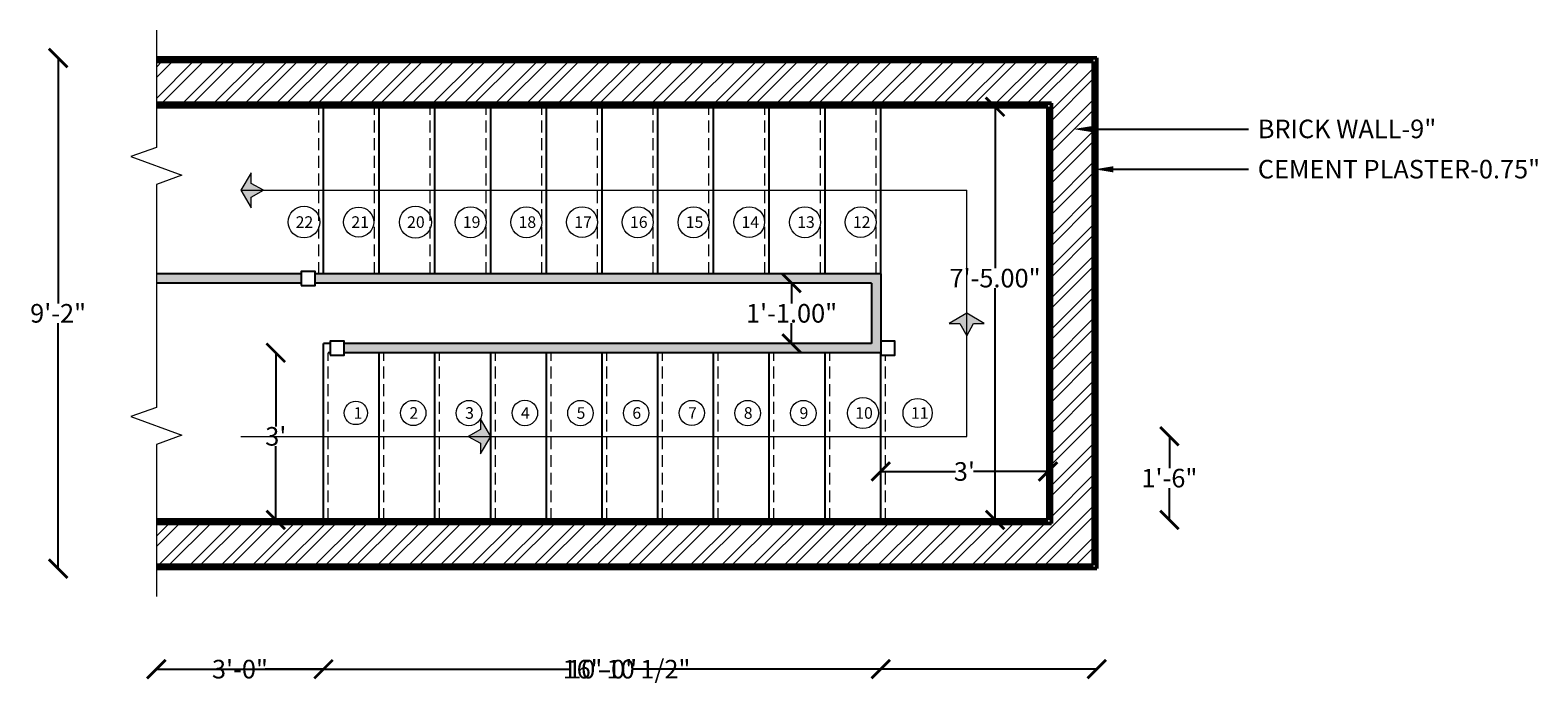
# Model space of a CAD drawing. Units: inches. Extents: x -27 to 693, y -28 to 216.
# Tile 1 of 2: x -27 to 298, y -28 to 116. Entities that reach past the tile are written whole.
import ezdxf
from ezdxf import colors
from ezdxf.entities.mleader import LeaderData, LeaderLine
from ezdxf.math import Vec2, Vec3

# ---------------------------------------------------------------- set-up
doc = ezdxf.new("R2010")
doc.units = ezdxf.units.IN
doc.linetypes.add('DASHED', pattern=[19.05, 12.7, -6.35])
for name, color, linetype, lineweight in [('A-ANNO-DIMS', 2, 'Continuous', 18), ('A-ANNO-SYMB', 3, 'Continuous', 18), ('A-ANNO-TEXT', 7, 'Continuous', 18), ('A-FLOR-HRAL', 4, 'Continuous', 25), ('A-FLOR-PATT', 8, 'Continuous', 13), ('A-FLOR-STRS', 1, 'Continuous', 25), ('A-FLOR-STRS-OVHD', 1, 'DASHED', 18), ('A-WALL', 7, 'Continuous', 50), ('A-WALL-PATT', 8, 'Continuous', 18)]:
    doc.layers.add(name, color=color, linetype=linetype, lineweight=lineweight)
doc.styles.get("Standard").update_dxf_attribs({"font": 'arial.ttf'})
doc.dimstyles.get("Standard").update_dxf_attribs({"dimtxt": 4, "dimasz": 4, "dimexe": 0.18, "dimexo": 0.0625, "dimgap": 0.09, "dimtad": 0, "dimtih": 1, "dimtoh": 1, "dimzin": 0, "dimdsep": 46, "dimlunit": 3, "dimtxsty": 'Standard', "dimblk": 'ARCHTICK', "dimcen": 0.09, "dimse1": 1, "dimse2": 1, "dimclrd": 4, "dimclrt": 2, "dimadec": 0, "dimazin": 0, "dimtfac": 1, "dimtofl": 0, "dimtmove": 0, "dimatfit": 3, "dimfxl": 1, "dimtolj": 1, "dimtzin": 0, "dimarcsym": 0})

# ---------------------------------------------------------------- blocks, each defined once
blk = doc.blocks.new('_ArchTick')
at = {"color": 0, "linetype": 'ByBlock', "const_width": 0.15}
blk.add_lwpolyline([(-0.5, -0.5), (0.5, 0.5)], dxfattribs=at)
blk = doc.blocks.new('*D3')
at = {"layer": 'A-ANNO-DIMS', "color": 0, "lineweight": -2, "transparency": 16777216}
for p, q in [((25.74, 46.24), (25.74, 30.37)), ((25.74, 10.24), (25.74, 26.1))]:
    blk.add_line(p, q, dxfattribs=at)
at = {"layer": 'DEFPOINTS', "color": 0, "transparency": 16777216}
for p in [(25.74, 46.24), (48.02, 46.24), (48.02, 10.24)]:
    blk.add_point(p, dxfattribs=at)
at = {"layer": 'A-ANNO-DIMS', "color": 0, "lineweight": -2, "transparency": 16777216, "xscale": 4, "yscale": 4, "zscale": 4}
for p, rotation in [((25.74, 46.24), 90), ((25.74, 10.24), 270)]:
    blk.add_blockref('_ArchTick', p, dxfattribs=dict(at, rotation=rotation))
at = {"layer": 'A-ANNO-DIMS', "color": 0, "transparency": 16777216, "insert": (25.74, 28.24), "char_height": 4, "attachment_point": 5}
blk.add_mtext("\\A1;3'", dxfattribs=at)
blk = doc.blocks.new('*D4')
at = {"layer": 'A-ANNO-DIMS', "color": 0, "lineweight": -2, "transparency": 16777216}
for p, q in [((136.81, 61.24), (136.81, 56.87)), ((136.81, 48.24), (136.81, 52.6))]:
    blk.add_line(p, q, dxfattribs=at)
at = {"layer": 'DEFPOINTS', "color": 0, "transparency": 16777216}
for p in [(154.02, 61.24), (136.81, 48.24), (154.02, 48.24)]:
    blk.add_point(p, dxfattribs=at)
at = {"layer": 'A-ANNO-DIMS', "color": 0, "lineweight": -2, "transparency": 16777216, "xscale": 4, "yscale": 4, "zscale": 4}
for p, rotation in [((136.81, 61.24), 90), ((136.81, 48.24), 270)]:
    blk.add_blockref('_ArchTick', p, dxfattribs=dict(at, rotation=rotation))
at = {"layer": 'A-ANNO-DIMS', "color": 0, "transparency": 16777216, "insert": (136.81, 54.74), "char_height": 4, "attachment_point": 5}
blk.add_mtext('\\A1;1\'-1.00"', dxfattribs=at)
blk = doc.blocks.new('*D5')
at = {"layer": 'A-ANNO-DIMS', "color": 0, "lineweight": -2, "transparency": 16777216}
for p, q in [((180.62, 99.24), (180.62, 64.45)), ((180.62, 10.24), (180.62, 60.18))]:
    blk.add_line(p, q, dxfattribs=at)
at = {"layer": 'DEFPOINTS', "color": 0, "transparency": 16777216}
for p in [(180.62, 99.24), (192.02, 99.24), (192.02, 10.24)]:
    blk.add_point(p, dxfattribs=at)
at = {"layer": 'A-ANNO-DIMS', "color": 0, "lineweight": -2, "transparency": 16777216, "xscale": 4, "yscale": 4, "zscale": 4}
for p, rotation in [((180.62, 99.24), 90), ((180.62, 10.24), 270)]:
    blk.add_blockref('_ArchTick', p, dxfattribs=dict(at, rotation=rotation))
at = {"layer": 'A-ANNO-DIMS', "color": 0, "transparency": 16777216, "insert": (180.62, 62.32), "char_height": 4, "attachment_point": 5}
blk.add_mtext('\\A1;7\'-5.00"', dxfattribs=at)
blk = doc.blocks.new('*D6')
at = {"layer": 'A-ANNO-DIMS', "color": 0, "lineweight": -2, "transparency": 16777216}
for p, q in [((156.02, 20.67), (172.09, 20.67)), ((192.02, 20.67), (175.95, 20.67))]:
    blk.add_line(p, q, dxfattribs=at)
at = {"layer": 'DEFPOINTS', "color": 0, "transparency": 16777216}
for p in [(192.02, 20.67), (156.02, 10.24), (192.02, 10.24)]:
    blk.add_point(p, dxfattribs=at)
at = {"layer": 'A-ANNO-DIMS', "color": 0, "lineweight": -2, "transparency": 16777216, "xscale": 4, "yscale": 4, "zscale": 4, "rotation": 180}
blk.add_blockref('_ArchTick', (156.02, 20.67), dxfattribs=at)
at = {"layer": 'A-ANNO-DIMS', "color": 0, "lineweight": -2, "transparency": 16777216, "xscale": 4, "yscale": 4, "zscale": 4}
blk.add_blockref('_ArchTick', (192.02, 20.67), dxfattribs=at)
at = {"layer": 'A-ANNO-DIMS', "color": 0, "transparency": 16777216, "insert": (174.02, 20.67), "char_height": 4, "attachment_point": 5}
blk.add_mtext("\\A1;3'", dxfattribs=at)
blk = doc.blocks.new('*D11')
at = {"layer": 'A-ANNO-DIMS', "color": 4, "lineweight": -2, "transparency": 16777216}
for p, q in [((0.02, -21.91), (88.28, -21.91)), ((202.52, -21.91), (114.25, -21.91))]:
    blk.add_line(p, q, dxfattribs=at)
at = {"layer": 'DEFPOINTS', "color": 0, "transparency": 16777216}
for p in [(0.02, -0.26), (202.52, -0.26), (202.52, -21.91)]:
    blk.add_point(p, dxfattribs=at)
at = {"layer": 'A-ANNO-DIMS', "color": 4, "lineweight": -2, "transparency": 16777216, "xscale": 4, "yscale": 4, "zscale": 4, "rotation": 180}
blk.add_blockref('_ArchTick', (0.02, -21.91), dxfattribs=at)
at = {"layer": 'A-ANNO-DIMS', "color": 4, "lineweight": -2, "transparency": 16777216, "xscale": 4, "yscale": 4, "zscale": 4}
blk.add_blockref('_ArchTick', (202.52, -21.91), dxfattribs=at)
at = {"layer": 'A-ANNO-DIMS', "color": 2, "transparency": 16777216, "insert": (101.27, -21.91), "char_height": 4, "attachment_point": 5}
blk.add_mtext('\\A1;16\'-10 1/2"', dxfattribs=at)
blk = doc.blocks.new('*D12')
at = {"layer": 'A-ANNO-DIMS', "color": 4, "lineweight": -2, "transparency": 16777216}
for p, q in [((0.02, -21.91), (12.61, -21.91)), ((36.02, -21.91), (23.42, -21.91))]:
    blk.add_line(p, q, dxfattribs=at)
at = {"layer": 'DEFPOINTS', "color": 0, "transparency": 16777216}
for p in [(0.02, 10.24), (36.02, 10.24), (36.02, -21.91)]:
    blk.add_point(p, dxfattribs=at)
at = {"layer": 'A-ANNO-DIMS', "color": 4, "lineweight": -2, "transparency": 16777216, "xscale": 4, "yscale": 4, "zscale": 4, "rotation": 180}
blk.add_blockref('_ArchTick', (0.02, -21.91), dxfattribs=at)
at = {"layer": 'A-ANNO-DIMS', "color": 4, "lineweight": -2, "transparency": 16777216, "xscale": 4, "yscale": 4, "zscale": 4}
blk.add_blockref('_ArchTick', (36.02, -21.91), dxfattribs=at)
at = {"layer": 'A-ANNO-DIMS', "color": 2, "transparency": 16777216, "insert": (18.02, -21.91), "char_height": 4, "attachment_point": 5}
blk.add_mtext('\\A1;3\'-0"', dxfattribs=at)
blk = doc.blocks.new('*D13')
at = {"layer": 'A-ANNO-DIMS', "color": 4, "lineweight": -2, "transparency": 16777216}
for p, q in [((36.02, -21.91), (89.24, -21.91)), ((156.02, -21.91), (102.79, -21.91))]:
    blk.add_line(p, q, dxfattribs=at)
at = {"layer": 'DEFPOINTS', "color": 0, "transparency": 16777216}
for p in [(36.02, 10.24), (156.02, 10.24), (156.02, -21.91)]:
    blk.add_point(p, dxfattribs=at)
at = {"layer": 'A-ANNO-DIMS', "color": 4, "lineweight": -2, "transparency": 16777216, "xscale": 4, "yscale": 4, "zscale": 4, "rotation": 180}
blk.add_blockref('_ArchTick', (36.02, -21.91), dxfattribs=at)
at = {"layer": 'A-ANNO-DIMS', "color": 4, "lineweight": -2, "transparency": 16777216, "xscale": 4, "yscale": 4, "zscale": 4}
blk.add_blockref('_ArchTick', (156.02, -21.91), dxfattribs=at)
at = {"layer": 'A-ANNO-DIMS', "color": 2, "transparency": 16777216, "insert": (96.02, -21.91), "char_height": 4, "attachment_point": 5}
blk.add_mtext('\\A1;10\'-0"', dxfattribs=at)
blk = doc.blocks.new('*D14')
at = {"layer": 'A-ANNO-DIMS', "color": 4, "lineweight": -2, "transparency": 16777216}
for p, q in [((-21.13, 109.74), (-21.13, 56.87)), ((-21.13, -0.26), (-21.13, 52.6))]:
    blk.add_line(p, q, dxfattribs=at)
at = {"layer": 'DEFPOINTS', "color": 0, "transparency": 16777216}
for p in [(-21.13, 109.74), (0.02, 109.74), (0.02, -0.26)]:
    blk.add_point(p, dxfattribs=at)
at = {"layer": 'A-ANNO-DIMS', "color": 4, "lineweight": -2, "transparency": 16777216, "xscale": 4, "yscale": 4, "zscale": 4}
for p, rotation in [((-21.13, 109.74), 90), ((-21.13, -0.26), 270)]:
    blk.add_blockref('_ArchTick', p, dxfattribs=dict(at, rotation=rotation))
at = {"layer": 'A-ANNO-DIMS', "color": 2, "transparency": 16777216, "insert": (-21.13, 54.74), "char_height": 4, "attachment_point": 5}
blk.add_mtext('\\A1;9\'-2"', dxfattribs=at)
blk = doc.blocks.new('*D15')
at = {"layer": 'A-ANNO-DIMS', "color": 4, "lineweight": -2, "transparency": 16777216}
for p, q in [((218.17, 28.24), (218.17, 21.37)), ((218.17, 10.24), (218.17, 17.1))]:
    blk.add_line(p, q, dxfattribs=at)
at = {"layer": 'DEFPOINTS', "color": 0, "transparency": 16777216}
for p in [(174.52, 28.24), (192.02, 10.24), (218.17, 10.24)]:
    blk.add_point(p, dxfattribs=at)
at = {"layer": 'A-ANNO-DIMS', "color": 4, "lineweight": -2, "transparency": 16777216, "xscale": 4, "yscale": 4, "zscale": 4}
for p, rotation in [((218.17, 28.24), 90), ((218.17, 10.24), 270)]:
    blk.add_blockref('_ArchTick', p, dxfattribs=dict(at, rotation=rotation))
at = {"layer": 'A-ANNO-DIMS', "color": 2, "transparency": 16777216, "insert": (218.17, 19.24), "char_height": 4, "attachment_point": 5}
blk.add_mtext('\\A1;1\'-6"', dxfattribs=at)

msp = doc.modelspace()

# ---------------------------------------------------------------- hatches: boundary and pattern name
at = {"layer": 'A-ANNO-SYMB'}
h = msp.add_hatch(color=256, dxfattribs=at)
h.dxf.hatch_style = 1
h.paths.add_polyline_path([(20.411, 77.497), (20.411, 79.771), (23.089, 81.237), (18.209, 81.237)])
h.paths.add_polyline_path([(18.209, 81.237), (23.089, 81.237), (20.411, 82.703), (20.411, 84.977)])
h = msp.add_hatch(color=256, dxfattribs=at)
h.dxf.hatch_style = 1
h.paths.add_polyline_path([(170.776, 52.535), (173.051, 52.535), (174.517, 49.857), (174.517, 54.737)])
h.paths.add_polyline_path([(174.517, 54.737), (174.517, 49.857), (175.982, 52.535), (178.257, 52.535)])
h = msp.add_hatch(color=256, dxfattribs=at)
h.dxf.hatch_style = 1
h.paths.add_polyline_path([(69.814, 31.977), (69.814, 29.703), (67.136, 28.237), (72.017, 28.237)])
h.paths.add_polyline_path([(72.017, 28.237), (67.136, 28.237), (69.814, 26.771), (69.814, 24.497)])
at = {"layer": 'A-FLOR-PATT'}
h = msp.add_hatch(dxfattribs=at)
h.set_pattern_fill('GOST_GLASS', color=256, scale=0.2)
h.paths.add_polyline_path([(156.017, 63.237), (34.183, 63.237), (34.183, 61.237), (154.017, 61.237), (154.017, 48.237), (40.433, 48.237), (40.433, 46.237), (156.017, 46.237)])
h.paths.add_polyline_path([(31.183, 63.237), (0.017, 63.237), (0.017, 61.237), (31.183, 61.237)])
at = {"layer": 'A-WALL-PATT'}
h = msp.add_hatch(dxfattribs=at)
h.set_pattern_fill('AR-CONC', color=256, scale=0.01)
h.paths.add_polyline_path([(192.767, 99.987), (0.017, 99.987), (0.017, 99.237), (192.017, 99.237), (192.017, 10.237), (0.017, 10.237), (0.017, 9.487), (192.767, 9.487)], flags=17)
h.paths.add_polyline_path([(202.517, 109.737), (0.017, 109.737), (0.017, 108.987), (201.767, 108.987), (201.767, 0.487), (0.017, 0.487), (0.017, -0.263), (202.517, -0.263)])
h = msp.add_hatch(dxfattribs=at)
h.set_pattern_fill('ANSI32', color=256, scale=0.5)
h.paths.add_polyline_path([(201.767, 108.987), (0.017, 108.987), (0.017, 99.987), (192.767, 99.987), (192.767, 9.487), (0.017, 9.487), (0.017, 0.487), (201.767, 0.487)])

# ---------------------------------------------------------------- linework, layer by layer
at = {"layer": 'A-ANNO-SYMB'}
for p, q in [((18.209, 81.237), (174.517, 81.237)), ((174.517, 28.237), (174.517, 81.237)), ((18.209, 28.237), (174.517, 28.237))]:
    msp.add_line(p, q, dxfattribs=at)
for points in [[(0.017, 115.737), (0.017, 90.487), (-5.478, 88.487), (5.512, 84.487), (0.017, 82.487), (0.017, 57.237)], [(0.017, 67.237), (0.017, 34.487), (-5.478, 32.487), (5.512, 28.487), (0.017, 26.487), (0.017, -6.263)]]:
    msp.add_lwpolyline(points, dxfattribs=at)
for points in [[(23.089, 81.237), (20.411, 82.703), (20.411, 84.977), (18.209, 81.237), (20.411, 77.497), (20.411, 79.771)], [(174.517, 49.857), (175.982, 52.535), (178.257, 52.535), (174.517, 54.737), (170.776, 52.535), (173.051, 52.535)], [(67.136, 28.237), (69.814, 26.771), (69.814, 24.497), (72.017, 28.237), (69.814, 31.977), (69.814, 29.703)]]:
    msp.add_lwpolyline(points, close=True, dxfattribs=at)
for centre, radius in [((31.816, 74.385), 3.419), ((43.587, 74.385), 3.243), ((55.824, 74.364), 3.439), ((67.692, 74.364), 3.337), ((79.692, 74.364), 3.337), ((91.69, 74.385), 3.321), ((103.689, 74.364), 3.334), ((115.699, 74.364), 3.342), ((127.684, 74.385), 3.317), ((139.69, 74.363), 3.335), ((151.677, 74.385), 3.311), ((42.977, 33.268), 2.514), ((55.345, 33.268), 2.727), ((67.335, 33.246), 2.739), ((79.381, 33.273), 2.746), ((91.345, 33.252), 2.74), ((103.342, 33.246), 2.742), ((115.326, 33.273), 2.711), ((127.34, 33.246), 2.741), ((139.339, 33.246), 2.74), ((152.185, 33.246), 3.331), ((163.948, 33.268), 3.14)]:
    msp.add_circle(centre, radius, dxfattribs=at)
at = {"layer": 'A-FLOR-HRAL'}
for p, q in [((31.183, 63.237), (0.017, 63.237)), ((156.017, 63.237), (34.183, 63.237)), ((156.017, 63.237), (156.017, 46.237)), ((31.183, 61.237), (0.017, 61.237)), ((154.017, 61.237), (34.183, 61.237)), ((154.017, 61.237), (154.017, 48.237)), ((37.433, 48.237), (36.017, 48.237)), ((37.433, 46.237), (37.017, 46.237)), ((154.017, 48.237), (40.433, 48.237)), ((156.017, 46.237), (40.433, 46.237))]:
    msp.add_line(p, q, dxfattribs=at)
for points in [[(31.183, 60.737), (34.183, 60.737), (34.183, 63.737), (31.183, 63.737)], [(37.433, 45.737), (40.433, 45.737), (40.433, 48.737), (37.433, 48.737)], [(156.017, 45.737), (159.017, 45.737), (159.017, 48.737), (156.017, 48.737)]]:
    msp.add_lwpolyline(points, close=True, dxfattribs=at)
at = {"layer": 'A-FLOR-STRS'}
for p, q in [((36.017, 63.237), (36.017, 99.237)), ((48.017, 63.237), (48.017, 99.237)), ((60.017, 63.237), (60.017, 99.237)), ((72.017, 63.237), (72.017, 99.237)), ((84.017, 63.237), (84.017, 99.237)), ((96.017, 63.237), (96.017, 99.237)), ((108.017, 63.237), (108.017, 99.237)), ((120.017, 63.237), (120.017, 99.237)), ((132.017, 63.237), (132.017, 99.237)), ((144.017, 63.237), (144.017, 99.237)), ((156.017, 63.237), (156.017, 99.237)), ((36.017, 10.237), (36.017, 48.237)), ((48.017, 10.237), (48.017, 46.237)), ((60.017, 10.237), (60.017, 46.237)), ((72.017, 10.237), (72.017, 46.237)), ((84.017, 10.237), (84.017, 46.237)), ((96.017, 10.237), (96.017, 46.237)), ((108.017, 10.237), (108.017, 46.237)), ((120.017, 10.237), (120.017, 46.237)), ((132.017, 10.237), (132.017, 46.237)), ((144.017, 10.237), (144.017, 46.237)), ((156.017, 10.237), (156.017, 46.237)), ((156.017, 10.237), (156.017, 46.237))]:
    msp.add_line(p, q, dxfattribs=at)
at = {"layer": 'A-FLOR-STRS-OVHD', "ltscale": 0.2}
for p, q in [((35.017, 63.237), (35.017, 99.237)), ((47.017, 63.237), (47.017, 99.237)), ((59.017, 63.237), (59.017, 99.237)), ((71.017, 63.237), (71.017, 99.237)), ((83.017, 63.237), (83.017, 99.237)), ((95.017, 63.237), (95.017, 99.237)), ((107.017, 63.237), (107.017, 99.237)), ((119.017, 63.237), (119.017, 99.237)), ((131.017, 63.237), (131.017, 99.237)), ((143.017, 63.237), (143.017, 99.237)), ((155.017, 63.237), (155.017, 99.237)), ((37.017, 10.237), (37.017, 46.237)), ((49.017, 10.237), (49.017, 46.237)), ((61.017, 10.237), (61.017, 46.237)), ((73.017, 10.237), (73.017, 46.237)), ((85.017, 10.237), (85.017, 46.237)), ((97.017, 10.237), (97.017, 46.237)), ((109.017, 10.237), (109.017, 46.237)), ((121.017, 10.237), (121.017, 46.237)), ((133.017, 10.237), (133.017, 46.237)), ((145.017, 10.237), (145.017, 46.237)), ((157.017, 10.237), (157.017, 45.737))]:
    msp.add_line(p, q, dxfattribs=at)
at = {"layer": 'A-WALL'}
for p, q in [((202.517, 109.737), (0.017, 109.737)), ((201.767, 108.987), (0.017, 108.987)), ((201.767, 0.487), (201.767, 108.987)), ((202.517, -0.263), (202.517, 109.737)), ((192.767, 99.987), (0.017, 99.987)), ((192.017, 99.237), (0.017, 99.237)), ((192.017, 10.237), (192.017, 99.237)), ((192.767, 9.487), (192.767, 99.987)), ((192.017, 10.237), (0.017, 10.237)), ((192.767, 9.487), (0.017, 9.487)), ((201.767, 0.487), (0.017, 0.487)), ((202.517, -0.263), (0.017, -0.263))]:
    msp.add_line(p, q, dxfattribs=at)

# ---------------------------------------------------------------- texts
at = {"layer": 'A-ANNO-TEXT', "char_height": 2.5, "attachment_point": 1}
for s, insert in [('22', (30.017, 75.64)), ('21', (42.017, 75.64)), ('20', (54.017, 75.64)), ('19', (66.017, 75.64)), ('18', (78.017, 75.64)), ('17', (90.017, 75.64)), ('16', (102.017, 75.64)), ('15', (114.017, 75.64)), ('14', (126.017, 75.64)), ('13', (138.017, 75.64)), ('12', (150.017, 75.64)), ('1', (42.517, 34.523)), ('2', (54.517, 34.523)), ('3', (66.517, 34.523)), ('4', (78.517, 34.523)), ('5', (90.517, 34.523)), ('6', (102.517, 34.523)), ('7', (114.517, 34.523)), ('8', (126.517, 34.523)), ('9', (138.517, 34.523)), ('10', (150.517, 34.523)), ('11', (162.517, 34.523))]:
    msp.add_mtext_dynamic_manual_height_columns(s, width=4.82371, gutter_width=12.5, heights=[0], dxfattribs=dict(at, insert=insert))

# ---------------------------------------------------------------- dimensions: what is measured, and where the dimension line sits
at = {"layer": 'A-ANNO-DIMS'}
for base, p1, p2, override, picture, middle in [((-21.128, 109.737), (0.017, -0.263), (0.017, 109.737), {"dimdec": 1, "dimlfac": 1, "dimrnd": 0, "dimzin": 1, "dimdsep": 46, "dimlunit": 4, "dimfrac": 2}, '*D14', (-21.128, 54.737)), ((136.807, 48.237), (154.017, 61.237), (154.017, 48.237), {"dimclrd": 0, "dimclre": 0, "dimclrt": 0}, '*D4', (136.807, 54.737)), ((25.74, 46.237), (48.017, 10.237), (48.017, 46.237), {"dimclrd": 0, "dimclre": 0, "dimclrt": 0}, '*D3', (25.74, 28.237)), ((218.167, 10.237), (174.517, 28.237), (192.017, 10.237), {"dimdec": 1, "dimlfac": 1, "dimrnd": 0, "dimzin": 1, "dimdsep": 46, "dimlunit": 4, "dimfrac": 2}, '*D15', (218.167, 19.237))]:
    dim = msp.add_linear_dim(base=base, p1=p1, p2=p2, angle=90, dimstyle='Standard', override=override, dxfattribs=at)
    dim.commit()
    dim.dimension.update_dxf_attribs({"geometry": picture, "text_midpoint": middle})
dim = msp.add_linear_dim(base=(180.622, 99.237), p1=(192.017, 10.237), p2=(192.017, 99.237), angle=90, dimstyle='Standard', override={"dimclrd": 0, "dimclre": 0, "dimclrt": 0}, dxfattribs=at)
dim.commit()
dim.dimension.update_dxf_attribs({"geometry": '*D5', "text_midpoint": (180.622, 62.316), "dimtype": 160})
for base, p1, p2, override, picture, middle in [((192.017, 20.673), (156.017, 10.237), (192.017, 10.237), {"dimclrd": 0, "dimclre": 0, "dimclrt": 0}, '*D6', (174.017, 20.673)), ((36.017, -21.913), (0.017, 10.237), (36.017, 10.237), {"dimdec": 1, "dimlfac": 1, "dimrnd": 0, "dimzin": 1, "dimdsep": 46, "dimlunit": 4, "dimfrac": 2}, '*D12', (18.017, -21.913)), ((156.017, -21.913), (36.017, 10.237), (156.017, 10.237), {"dimdec": 1, "dimlfac": 1, "dimrnd": 0, "dimzin": 1, "dimdsep": 46, "dimlunit": 4, "dimfrac": 2}, '*D13', (96.017, -21.913)), ((202.517, -21.913), (0.017, -0.263), (202.517, -0.263), {"dimdec": 1, "dimlfac": 1, "dimrnd": 0, "dimzin": 1, "dimdsep": 46, "dimlunit": 4, "dimfrac": 2}, '*D11', (101.267, -21.913))]:
    dim = msp.add_linear_dim(base=base, p1=p1, p2=p2, dimstyle='Standard', override=override, dxfattribs=at)
    dim.commit()
    dim.dimension.update_dxf_attribs({"geometry": picture, "text_midpoint": middle})

# ---------------------------------------------------------------- leaders
at = {"layer": 'A-ANNO-TEXT'}
ml = msp.add_multileader_mtext('Standard', dxfattribs=at)
ml.set_content('BRICK WALL-9"', color=256)
ml.set_leader_properties()
ml.build(insert=Vec2(0, 0))
ctx = ml.context
ctx.base_point, ctx.plane_origin = Vec3(235.208, 94.424), Vec3(197.523, 94.424)
notes = []
notes.append((ctx, [(0, (1, 1, 0), (227.208, 94.424), (1, 0), 8, [(0, [(197.523, 94.424)], 0, [])])]))
ctx.mtext.insert, ctx.mtext.flow_direction = Vec3(237.208, 96.458), 5
ml = msp.add_multileader_mtext('Standard', dxfattribs=at)
ml.set_content('CEMENT PLASTER-0.75"', color=256)
ml.set_leader_properties()
ml.build(insert=Vec2(0, 0))
ctx = ml.context
ctx.base_point, ctx.plane_origin = Vec3(235.208, 85.76), Vec3(202.059, 85.76)
notes.append((ctx, [(0, (1, 1, 0), (227.208, 85.76), (1, 0), 8, [(0, [(202.059, 85.76)], 0, [])])]))
ctx.mtext.insert, ctx.mtext.flow_direction = Vec3(237.208, 87.794), 5
for ctx, leaders in notes:
    for number, flags, end, landing, length, lines in leaders:
        leader = LeaderData()
        leader.index, (leader.has_last_leader_line, leader.has_dogleg_vector, leader.attachment_direction) = number, flags
        leader.last_leader_point, leader.dogleg_vector, leader.dogleg_length = Vec3(end), Vec3(landing), length
        for number, points, colour, breaks in lines:
            line = LeaderLine()
            line.index, line.vertices, line.color, line.breaks = number, Vec3.list(points), colors.encode_raw_color(colour), breaks
            leader.lines.append(line)
        ctx.leaders.append(leader)

doc.saveas('drawing.dxf')
